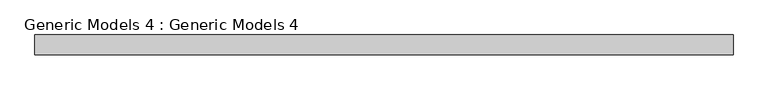
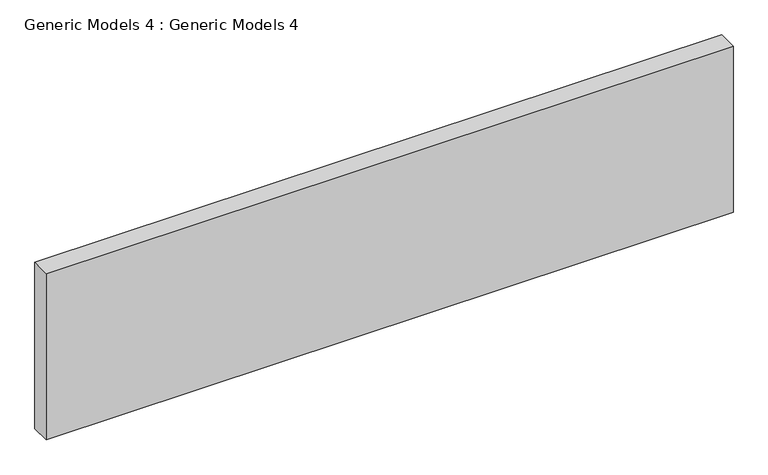
"""IFC4 building model written with IfcOpenShell, lengths in millimetres: proxy geometry, Generic Models 4 : Generic Models 4."""

from ifc_helpers import new_model, si_unit, frame, origin, place, context, project, spatial, polyline, outline, extrude, source, transform, mapped, element, save


def generic_models_4_generic_models_4_98a53d0d(model_context):
    return source(origin(), model_context, "Body", "SweptSolid", [
        extrude(outline(polyline([(-8399.3906521, -11669.8453012), (-11970.3047236, -11669.8453012), (-11970.3047236, -11568.2453012), (-8399.3906521, -11568.2453012), (-8399.3906521, -11669.8453012)])), frame((0.0, 0.0, 6096.0), z_axis=(0.0, 0.0, 1.0), x_axis=(1.0, 0.0, 0.0)), (0.0, 0.0, 1.0), 914.4),
    ])


if __name__ == "__main__":
    model = new_model("IFC4")
    model_context = context("Model", 3, world=origin())
    ifc_project = project(units=[si_unit("LENGTHUNIT", "METRE", prefix="MILLI")], contexts=[model_context])
    site = spatial("IfcSite", under=ifc_project)
    building = spatial("IfcBuilding", under=site)
    placement = place(None, origin())
    generic_models_4_generic_models_4_shape = generic_models_4_generic_models_4_98a53d0d(model_context)
    element("IfcBuildingElementProxy", 1, Name="Generic Models 4 : Generic Models 4", ObjectType="Generic Models 4 : Generic Models 4", at=placement, inside=building, context=model_context, shape_type="MappedRepresentation", body=[
        mapped(generic_models_4_generic_models_4_shape, transform((0.0, 0.0, 0.0), x_axis=(1.0, 0.0, 0.0), y_axis=(0.0, 1.0, 0.0), z_axis=(0.0, 0.0, 1.0))),
    ])
    save(model, "model.ifc")
